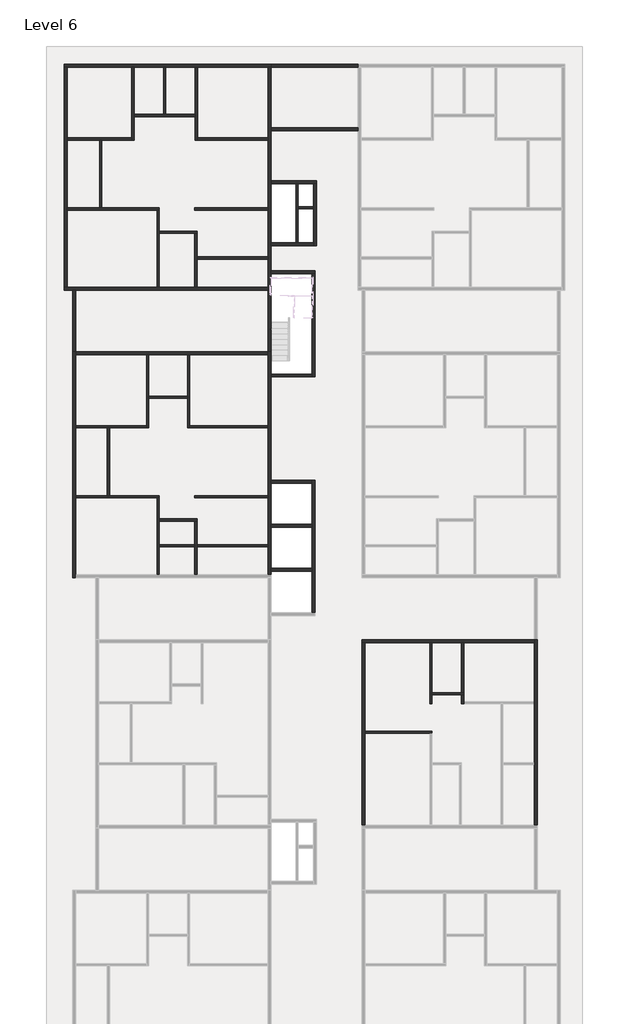
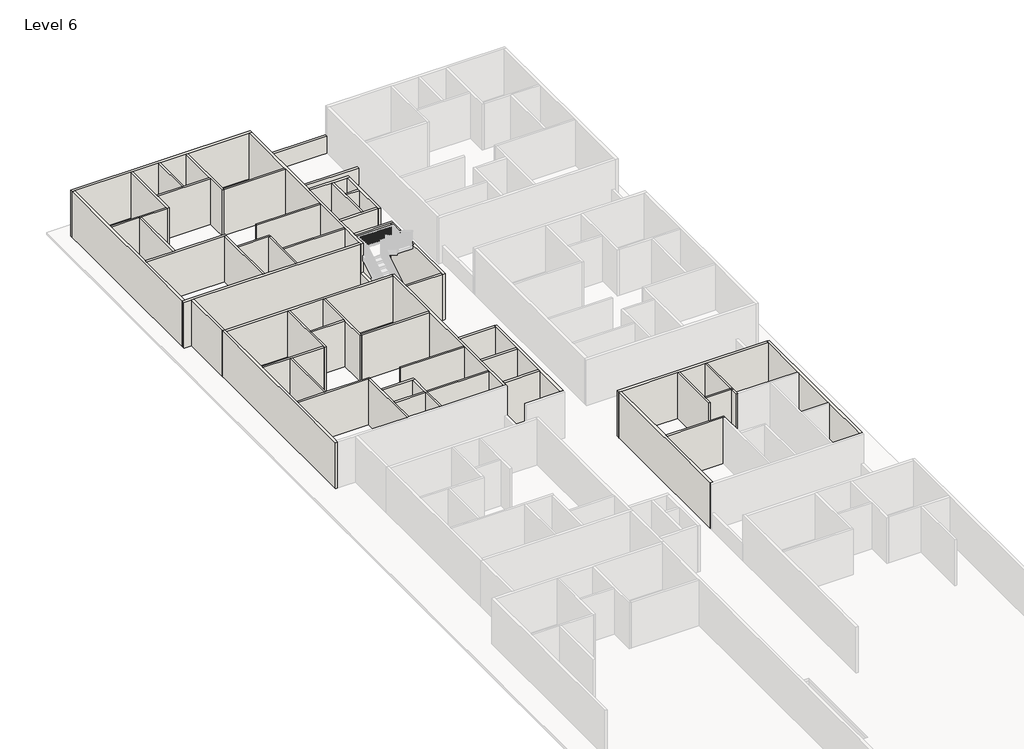
# One storey, part 3 of 8: 57 walls.
"""IFC4 building model written with IfcOpenShell, lengths in millimetres."""

from ifc_helpers import new_model, si_unit, frame, origin, place, context, project, spatial, polyline, outline, extrude, faceted_brep, element, save

model = new_model("IFC4")

# Units and contexts
model_context = context("Model", 3, world=origin())
ifc_project = project(units=[si_unit("LENGTHUNIT", "METRE", prefix="MILLI")], contexts=[model_context])

# Site, building, storey
site = spatial("IfcSite", under=ifc_project)
building = spatial("IfcBuilding", under=site)
storey = spatial("IfcBuildingStorey", under=building, Name="Level 6", Elevation=40474.6172466)

# Walls
placement = place(None, origin())
element("IfcWall", 1, ObjectType="4.5\"", at=placement, inside=storey, context=model_context, shape_type="Brep", body=[
    faceted_brep([(-10818.3415084, 35031.1216096, 40474.6172466), (-10818.3415084, 31373.5216096, 40474.6172466), (-10818.3415084, 31259.2216096, 40474.6172466), (-10818.3415084, 31259.2216096, 43522.6172466), (-10818.3415084, 31373.5216096, 43522.6172466), (-10818.3415084, 35031.1216096, 43522.6172466), (-10704.0415084, 35031.1216096, 40474.6172466), (-10704.0415084, 35031.1216096, 43522.6172466), (-10704.0415084, 32592.7216096, 43522.6172466), (-10704.0415084, 32478.4216096, 43522.6172466), (-10704.0415084, 31259.2216096, 43522.6172466), (-10704.0415084, 31259.2216096, 40474.6172466), (-10704.0415084, 32478.4216096, 40474.6172466), (-10704.0415084, 32592.7216096, 40474.6172466)], [[[0, 1, 2, 3, 4, 5]], [[6, 7, 8, 9, 10, 11, 12, 13]], [[2, 1, 0, 6, 13, 12, 11]], [[0, 5, 7, 6]], [[3, 2, 11, 10]], [[5, 4, 3, 10, 9, 8, 7]]]),
])
element("IfcWall", 2, ObjectType="4.5\"", at=placement, inside=storey, context=model_context, shape_type="Brep", body=[
    faceted_brep([(-10818.3415084, 31373.5216096, 40474.6172466), (-14171.1415084, 31373.5216096, 40474.6172466), (-14171.1415084, 31373.5216096, 43522.6172466), (-10818.3415084, 31373.5216096, 43522.6172466), (-10818.3415084, 31259.2216096, 40474.6172466), (-10818.3415084, 31259.2216096, 43522.6172466), (-12380.4415084, 31259.2216096, 43522.6172466), (-12494.7415084, 31259.2216096, 43522.6172466), (-14171.1415084, 31259.2216096, 43522.6172466), (-14171.1415084, 31259.2216096, 40474.6172466), (-12494.7415084, 31259.2216096, 40474.6172466), (-12380.4415084, 31259.2216096, 40474.6172466)], [[[0, 1, 2, 3]], [[4, 5, 6, 7, 8, 9, 10, 11]], [[1, 0, 4, 11, 10, 9]], [[0, 3, 5, 4]], [[2, 1, 9, 8]], [[3, 2, 8, 7, 6, 5]]]),
])
element("IfcWall", 3, ObjectType="4.5\"", at=placement, inside=storey, context=model_context, shape_type="SweptSolid", body=[
    extrude(outline(polyline([(-12494.7415084, 27754.0216096), (-12494.7415084, 31259.2216096), (-12380.4415084, 31259.2216096), (-12380.4415084, 27754.0216096), (-12494.7415084, 27754.0216096)])), frame((0.0, 0.0, 40474.6172466), z_axis=(0.0, 0.0, 1.0), x_axis=(1.0, 0.0, 0.0)), (0.0, 0.0, 1.0), 3048.0),
])
element("IfcWall", 4, ObjectType="4.5\"", at=placement, inside=storey, context=model_context, shape_type="Brep", body=[
    faceted_brep([(-14171.1415084, 27639.7216096, 40474.6172466), (-9510.2415084, 27639.7216096, 40474.6172466), (-9395.9415084, 27639.7216096, 40474.6172466), (-9395.9415084, 27639.7216096, 43522.6172466), (-9510.2415084, 27639.7216096, 43522.6172466), (-14171.1415084, 27639.7216096, 43522.6172466), (-14171.1415084, 27754.0216096, 40474.6172466), (-14171.1415084, 27754.0216096, 43522.6172466), (-12494.7415084, 27754.0216096, 43522.6172466), (-12380.4415084, 27754.0216096, 43522.6172466), (-9395.9415084, 27754.0216096, 43522.6172466), (-9395.9415084, 27754.0216096, 40474.6172466), (-12380.4415084, 27754.0216096, 40474.6172466), (-12494.7415084, 27754.0216096, 40474.6172466)], [[[0, 1, 2, 3, 4, 5]], [[6, 7, 8, 9, 10, 11, 12, 13]], [[2, 1, 0, 6, 13, 12, 11]], [[0, 5, 7, 6]], [[3, 2, 11, 10]], [[5, 4, 3, 10, 9, 8, 7]]]),
])
element("IfcWall", 5, ObjectType="4.5\"", at=placement, inside=storey, context=model_context, shape_type="Brep", body=[
    faceted_brep([(-9510.2415084, 27639.7216096, 40474.6172466), (-9510.2415084, 23651.9216096, 40474.6172466), (-9510.2415084, 23651.9216096, 43522.6172466), (-9510.2415084, 27639.7216096, 43522.6172466), (-9395.9415084, 27639.7216096, 40474.6172466), (-9395.9415084, 27639.7216096, 43522.6172466), (-9395.9415084, 26547.5216096, 43522.6172466), (-9395.9415084, 26433.2216096, 43522.6172466), (-9395.9415084, 23651.9216096, 43522.6172466), (-9395.9415084, 23651.9216096, 40474.6172466), (-9395.9415084, 26433.2216096, 40474.6172466), (-9395.9415084, 26547.5216096, 40474.6172466)], [[[0, 1, 2, 3]], [[4, 5, 6, 7, 8, 9, 10, 11]], [[1, 0, 4, 11, 10, 9]], [[0, 3, 5, 4]], [[2, 1, 9, 8]], [[3, 2, 8, 7, 6, 5]]]),
])
element("IfcWall", 6, ObjectType="4.5\"", at=placement, inside=storey, context=model_context, shape_type="Brep", body=[
    faceted_brep([(-9395.9415084, 26433.2216096, 40474.6172466), (-7567.1415084, 26433.2216096, 40474.6172466), (-7452.8415084, 26433.2216096, 40474.6172466), (-7452.8415084, 26433.2216096, 43522.6172466), (-7567.1415084, 26433.2216096, 43522.6172466), (-9395.9415084, 26433.2216096, 43522.6172466), (-9395.9415084, 26547.5216096, 40474.6172466), (-9395.9415084, 26547.5216096, 43522.6172466), (-7452.8415084, 26547.5216096, 43522.6172466), (-7452.8415084, 26547.5216096, 40474.6172466)], [[[0, 1, 2, 3, 4, 5]], [[6, 7, 8, 9]], [[2, 1, 0, 6, 9]], [[0, 5, 7, 6]], [[3, 2, 9, 8]], [[5, 4, 3, 8, 7]]]),
])
element("IfcWall", 7, ObjectType="4.5\"", at=placement, inside=storey, context=model_context, shape_type="Brep", body=[
    faceted_brep([(-7567.1415084, 26433.2216096, 40474.6172466), (-7567.1415084, 23651.9216096, 40474.6172466), (-7567.1415084, 23651.9216096, 43522.6172466), (-7567.1415084, 26433.2216096, 43522.6172466), (-7452.8415084, 26433.2216096, 40474.6172466), (-7452.8415084, 26433.2216096, 43522.6172466), (-7452.8415084, 25214.0216096, 43522.6172466), (-7452.8415084, 25099.7216096, 43522.6172466), (-7452.8415084, 23651.9216096, 43522.6172466), (-7452.8415084, 23651.9216096, 40474.6172466), (-7452.8415084, 25099.7216096, 40474.6172466), (-7452.8415084, 25214.0216096, 40474.6172466)], [[[0, 1, 2, 3]], [[4, 5, 6, 7, 8, 9, 10, 11]], [[1, 0, 4, 11, 10, 9]], [[0, 3, 5, 4]], [[2, 1, 9, 8]], [[3, 2, 8, 7, 6, 5]]]),
])
element("IfcWall", 8, ObjectType="4.5\"", at=placement, inside=storey, context=model_context, shape_type="SweptSolid", body=[
    extrude(outline(polyline([(-7452.8415084, 25214.0216096), (-3769.8415084, 25214.0216096), (-3769.8415084, 25099.7216096), (-7452.8415084, 25099.7216096), (-7452.8415084, 25214.0216096)])), frame((0.0, 0.0, 40474.6172466), z_axis=(0.0, 0.0, 1.0), x_axis=(1.0, 0.0, 0.0)), (0.0, 0.0, 1.0), 3048.0),
])
element("IfcWall", 9, ObjectType="4.5\"", at=placement, inside=storey, context=model_context, shape_type="SweptSolid", body=[
    extrude(outline(polyline([(-3769.8415084, 27639.7216096), (-7567.1415084, 27639.7216096), (-7567.1415084, 27754.0216096), (-3769.8415084, 27754.0216096), (-3769.8415084, 27639.7216096)])), frame((0.0, 0.0, 40474.6172466), z_axis=(0.0, 0.0, 1.0), x_axis=(1.0, 0.0, 0.0)), (0.0, 0.0, 1.0), 3048.0),
])
element("IfcWall", 10, ObjectType="4.5\"", at=placement, inside=storey, context=model_context, shape_type="Brep", body=[
    faceted_brep([(-10704.0415084, 32478.4216096, 40474.6172466), (-7541.7415084, 32478.4216096, 40474.6172466), (-7541.7415084, 32478.4216096, 43522.6172466), (-10704.0415084, 32478.4216096, 43522.6172466), (-10704.0415084, 32592.7216096, 40474.6172466), (-10704.0415084, 32592.7216096, 43522.6172466), (-9180.0415084, 32592.7216096, 43522.6172466), (-9065.7415084, 32592.7216096, 43522.6172466), (-7541.7415084, 32592.7216096, 43522.6172466), (-7541.7415084, 32592.7216096, 40474.6172466), (-9065.7415084, 32592.7216096, 40474.6172466), (-9180.0415084, 32592.7216096, 40474.6172466)], [[[0, 1, 2, 3]], [[4, 5, 6, 7, 8, 9, 10, 11]], [[1, 0, 4, 11, 10, 9]], [[0, 3, 5, 4]], [[2, 1, 9, 8]], [[3, 2, 8, 7, 6, 5]]]),
])
element("IfcWall", 11, ObjectType="4.5\"", at=placement, inside=storey, context=model_context, shape_type="SweptSolid", body=[
    extrude(outline(polyline([(-9180.0415084, 32592.7216096), (-9180.0415084, 35031.1216096), (-9065.7415084, 35031.1216096), (-9065.7415084, 32592.7216096), (-9180.0415084, 32592.7216096)])), frame((0.0, 0.0, 40474.6172466), z_axis=(0.0, 0.0, 1.0), x_axis=(1.0, 0.0, 0.0)), (0.0, 0.0, 1.0), 3048.0),
])
element("IfcWall", 12, ObjectType="4.5\"", at=placement, inside=storey, context=model_context, shape_type="Brep", body=[
    faceted_brep([(-7541.7415084, 35031.1216096, 40474.6172466), (-7541.7415084, 32592.7216096, 40474.6172466), (-7541.7415084, 32478.4216096, 40474.6172466), (-7541.7415084, 31259.2216096, 40474.6172466), (-7541.7415084, 31259.2216096, 43522.6172466), (-7541.7415084, 32478.4216096, 43522.6172466), (-7541.7415084, 32592.7216096, 43522.6172466), (-7541.7415084, 35031.1216096, 43522.6172466), (-7427.4415084, 35031.1216096, 40474.6172466), (-7427.4415084, 35031.1216096, 43522.6172466), (-7427.4415084, 31373.5216096, 43522.6172466), (-7427.4415084, 31259.2216096, 43522.6172466), (-7427.4415084, 31259.2216096, 40474.6172466), (-7427.4415084, 31373.5216096, 40474.6172466)], [[[0, 1, 2, 3, 4, 5, 6, 7]], [[8, 9, 10, 11, 12, 13]], [[3, 2, 1, 0, 8, 13, 12]], [[0, 7, 9, 8]], [[4, 3, 12, 11]], [[7, 6, 5, 4, 11, 10, 9]]]),
])
element("IfcWall", 13, ObjectType="4.5\"", at=placement, inside=storey, context=model_context, shape_type="SweptSolid", body=[
    extrude(outline(polyline([(-3769.8415084, 31259.2216096), (-7427.4415084, 31259.2216096), (-7427.4415084, 31373.5216096), (-3769.8415084, 31373.5216096), (-3769.8415084, 31259.2216096)])), frame((0.0, 0.0, 40474.6172466), z_axis=(0.0, 0.0, 1.0), x_axis=(1.0, 0.0, 0.0)), (0.0, 0.0, 1.0), 3048.0),
])
element("IfcWall", 14, ObjectType="4.5\"", at=placement, inside=storey, context=model_context, shape_type="Brep", body=[
    faceted_brep([(-10061.4044854, 20146.7216096, 40474.6172466), (-10061.4044854, 16489.1216096, 40474.6172466), (-10061.4044854, 16374.8216096, 40474.6172466), (-10061.4044854, 16374.8216096, 43522.6172466), (-10061.4044854, 16489.1216096, 43522.6172466), (-10061.4044854, 20146.7216096, 43522.6172466), (-9947.1044854, 20146.7216096, 40474.6172466), (-9947.1044854, 20146.7216096, 43522.6172466), (-9947.1044854, 18013.1216096, 43522.6172466), (-9947.1044854, 17898.8216096, 43522.6172466), (-9947.1044854, 16374.8216096, 43522.6172466), (-9947.1044854, 16374.8216096, 40474.6172466), (-9947.1044854, 17898.8216096, 40474.6172466), (-9947.1044854, 18013.1216096, 40474.6172466)], [[[0, 1, 2, 3, 4, 5]], [[6, 7, 8, 9, 10, 11, 12, 13]], [[2, 1, 0, 6, 13, 12, 11]], [[0, 5, 7, 6]], [[3, 2, 11, 10]], [[5, 4, 3, 10, 9, 8, 7]]]),
])
element("IfcWall", 15, ObjectType="4.5\"", at=placement, inside=storey, context=model_context, shape_type="Brep", body=[
    faceted_brep([(-10061.4044854, 16489.1216096, 40474.6172466), (-13719.0044854, 16489.1216096, 40474.6172466), (-13719.0044854, 16489.1216096, 43522.6172466), (-10061.4044854, 16489.1216096, 43522.6172466), (-10061.4044854, 16374.8216096, 40474.6172466), (-10061.4044854, 16374.8216096, 43522.6172466), (-11980.3915084, 16374.8216096, 43522.6172466), (-12094.6915084, 16374.8216096, 43522.6172466), (-13719.0044854, 16374.8216096, 43522.6172466), (-13719.0044854, 16374.8216096, 40474.6172466), (-12094.6915084, 16374.8216096, 40474.6172466), (-11980.3915084, 16374.8216096, 40474.6172466)], [[[0, 1, 2, 3]], [[4, 5, 6, 7, 8, 9, 10, 11]], [[1, 0, 4, 11, 10, 9]], [[0, 3, 5, 4]], [[2, 1, 9, 8]], [[3, 2, 8, 7, 6, 5]]]),
])
element("IfcWall", 16, ObjectType="4.5\"", at=placement, inside=storey, context=model_context, shape_type="SweptSolid", body=[
    extrude(outline(polyline([(-7940.5044854, 17898.8216096), (-9947.1044854, 17898.8216096), (-9947.1044854, 18013.1216096), (-7940.5044854, 18013.1216096), (-7940.5044854, 17898.8216096)])), frame((0.0, 0.0, 40474.6172466), z_axis=(0.0, 0.0, 1.0), x_axis=(1.0, 0.0, 0.0)), (0.0, 0.0, 1.0), 3048.0),
])
element("IfcWall", 17, ObjectType="4.5\"", at=placement, inside=storey, context=model_context, shape_type="Brep", body=[
    faceted_brep([(-7940.5044854, 20146.7216096, 40474.6172466), (-7940.5044854, 18013.1216096, 40474.6172466), (-7940.5044854, 17898.8216096, 40474.6172466), (-7940.5044854, 16374.8216096, 40474.6172466), (-7940.5044854, 16374.8216096, 43522.6172466), (-7940.5044854, 17898.8216096, 43522.6172466), (-7940.5044854, 18013.1216096, 43522.6172466), (-7940.5044854, 20146.7216096, 43522.6172466), (-7826.2044854, 20146.7216096, 40474.6172466), (-7826.2044854, 20146.7216096, 43522.6172466), (-7826.2044854, 16489.1216096, 43522.6172466), (-7826.2044854, 16374.8216096, 43522.6172466), (-7826.2044854, 16374.8216096, 40474.6172466), (-7826.2044854, 16489.1216096, 40474.6172466)], [[[0, 1, 2, 3, 4, 5, 6, 7]], [[8, 9, 10, 11, 12, 13]], [[3, 2, 1, 0, 8, 13, 12]], [[0, 7, 9, 8]], [[4, 3, 12, 11]], [[7, 6, 5, 4, 11, 10, 9]]]),
])
element("IfcWall", 18, ObjectType="4.5\"", at=placement, inside=storey, context=model_context, shape_type="SweptSolid", body=[
    extrude(outline(polyline([(-3769.8415084, 16374.8216096), (-7826.2044854, 16374.8216096), (-7826.2044854, 16489.1216096), (-3769.8415084, 16489.1216096), (-3769.8415084, 16374.8216096)])), frame((0.0, 0.0, 40474.6172466), z_axis=(0.0, 0.0, 1.0), x_axis=(1.0, 0.0, 0.0)), (0.0, 0.0, 1.0), 3048.0),
])
element("IfcWall", 19, ObjectType="4.5\"", at=placement, inside=storey, context=model_context, shape_type="SweptSolid", body=[
    extrude(outline(polyline([(-12094.6915084, 12869.6216096), (-12094.6915084, 16374.8216096), (-11980.3915084, 16374.8216096), (-11980.3915084, 12869.6216096), (-12094.6915084, 12869.6216096)])), frame((0.0, 0.0, 40474.6172466), z_axis=(0.0, 0.0, 1.0), x_axis=(1.0, 0.0, 0.0)), (0.0, 0.0, 1.0), 3048.0),
])
element("IfcWall", 20, ObjectType="4.5\"", at=placement, inside=storey, context=model_context, shape_type="Brep", body=[
    faceted_brep([(-13719.0044854, 12755.3216096, 40474.6172466), (-9510.2415084, 12755.3216096, 40474.6172466), (-9395.9415084, 12755.3216096, 40474.6172466), (-9395.9415084, 12755.3216096, 43522.6172466), (-9510.2415084, 12755.3216096, 43522.6172466), (-13719.0044854, 12755.3216096, 43522.6172466), (-13719.0044854, 12869.6216096, 40474.6172466), (-13719.0044854, 12869.6216096, 43522.6172466), (-12094.6915084, 12869.6216096, 43522.6172466), (-11980.3915084, 12869.6216096, 43522.6172466), (-9395.9415084, 12869.6216096, 43522.6172466), (-9395.9415084, 12869.6216096, 40474.6172466), (-11980.3915084, 12869.6216096, 40474.6172466), (-12094.6915084, 12869.6216096, 40474.6172466)], [[[0, 1, 2, 3, 4, 5]], [[6, 7, 8, 9, 10, 11, 12, 13]], [[2, 1, 0, 6, 13, 12, 11]], [[0, 5, 7, 6]], [[3, 2, 11, 10]], [[5, 4, 3, 10, 9, 8, 7]]]),
])
element("IfcWall", 21, ObjectType="4.5\"", at=placement, inside=storey, context=model_context, shape_type="Brep", body=[
    faceted_brep([(-9510.2415084, 12755.3216096, 40474.6172466), (-9510.2415084, 8767.5216096, 40474.6172466), (-9510.2415084, 8767.5216096, 43522.6172466), (-9510.2415084, 12755.3216096, 43522.6172466), (-9395.9415084, 12755.3216096, 40474.6172466), (-9395.9415084, 12755.3216096, 43522.6172466), (-9395.9415084, 11663.1216096, 43522.6172466), (-9395.9415084, 11548.8216096, 43522.6172466), (-9395.9415084, 10329.6216096, 43522.6172466), (-9395.9415084, 10215.3216096, 43522.6172466), (-9395.9415084, 8767.5216096, 43522.6172466), (-9395.9415084, 8767.5216096, 40474.6172466), (-9395.9415084, 10215.3216096, 40474.6172466), (-9395.9415084, 10329.6216096, 40474.6172466), (-9395.9415084, 11548.8216096, 40474.6172466), (-9395.9415084, 11663.1216096, 40474.6172466)], [[[0, 1, 2, 3]], [[4, 5, 6, 7, 8, 9, 10, 11, 12, 13, 14, 15]], [[1, 0, 4, 15, 14, 13, 12, 11]], [[0, 3, 5, 4]], [[2, 1, 11, 10]], [[3, 2, 10, 9, 8, 7, 6, 5]]]),
])
element("IfcWall", 22, ObjectType="4.5\"", at=placement, inside=storey, context=model_context, shape_type="SweptSolid", body=[
    extrude(outline(polyline([(-7567.1415084, 10215.3216096), (-9395.9415084, 10215.3216096), (-9395.9415084, 10329.6216096), (-7567.1415084, 10329.6216096), (-7567.1415084, 10215.3216096)])), frame((0.0, 0.0, 40474.6172466), z_axis=(0.0, 0.0, 1.0), x_axis=(1.0, 0.0, 0.0)), (0.0, 0.0, 1.0), 3048.0),
])
element("IfcWall", 23, ObjectType="4.5\"", at=placement, inside=storey, context=model_context, shape_type="Brep", body=[
    faceted_brep([(-9395.9415084, 11548.8216096, 40474.6172466), (-7567.1415084, 11548.8216096, 40474.6172466), (-7452.8415084, 11548.8216096, 40474.6172466), (-7452.8415084, 11548.8216096, 43522.6172466), (-7567.1415084, 11548.8216096, 43522.6172466), (-9395.9415084, 11548.8216096, 43522.6172466), (-9395.9415084, 11663.1216096, 40474.6172466), (-9395.9415084, 11663.1216096, 43522.6172466), (-7452.8415084, 11663.1216096, 43522.6172466), (-7452.8415084, 11663.1216096, 40474.6172466)], [[[0, 1, 2, 3, 4, 5]], [[6, 7, 8, 9]], [[2, 1, 0, 6, 9]], [[0, 5, 7, 6]], [[3, 2, 9, 8]], [[5, 4, 3, 8, 7]]]),
])
element("IfcWall", 24, ObjectType="4.5\"", at=placement, inside=storey, context=model_context, shape_type="Brep", body=[
    faceted_brep([(-7567.1415084, 11548.8216096, 40474.6172466), (-7567.1415084, 10329.6216096, 40474.6172466), (-7567.1415084, 10215.3216096, 40474.6172466), (-7567.1415084, 8767.5216096, 40474.6172466), (-7567.1415084, 8767.5216096, 43522.6172466), (-7567.1415084, 10215.3216096, 43522.6172466), (-7567.1415084, 10329.6216096, 43522.6172466), (-7567.1415084, 11548.8216096, 43522.6172466), (-7452.8415084, 11548.8216096, 40474.6172466), (-7452.8415084, 11548.8216096, 43522.6172466), (-7452.8415084, 10329.6216096, 43522.6172466), (-7452.8415084, 10215.3216096, 43522.6172466), (-7452.8415084, 8767.5216096, 43522.6172466), (-7452.8415084, 8767.5216096, 40474.6172466), (-7452.8415084, 10215.3216096, 40474.6172466), (-7452.8415084, 10329.6216096, 40474.6172466)], [[[0, 1, 2, 3, 4, 5, 6, 7]], [[8, 9, 10, 11, 12, 13, 14, 15]], [[3, 2, 1, 0, 8, 15, 14, 13]], [[0, 7, 9, 8]], [[4, 3, 13, 12]], [[7, 6, 5, 4, 12, 11, 10, 9]]]),
])
element("IfcWall", 25, ObjectType="4.5\"", at=placement, inside=storey, context=model_context, shape_type="SweptSolid", body=[
    extrude(outline(polyline([(-3769.8415084, 10215.3216096), (-7452.8415084, 10215.3216096), (-7452.8415084, 10329.6216096), (-3769.8415084, 10329.6216096), (-3769.8415084, 10215.3216096)])), frame((0.0, 0.0, 40474.6172466), z_axis=(0.0, 0.0, 1.0), x_axis=(1.0, 0.0, 0.0)), (0.0, 0.0, 1.0), 3048.0),
])
element("IfcWall", 26, ObjectType="4.5\"", at=placement, inside=storey, context=model_context, shape_type="SweptSolid", body=[
    extrude(outline(polyline([(-3769.8415084, 12755.3216096), (-7567.1415084, 12755.3216096), (-7567.1415084, 12869.6216096), (-3769.8415084, 12869.6216096), (-3769.8415084, 12755.3216096)])), frame((0.0, 0.0, 40474.6172466), z_axis=(0.0, 0.0, 1.0), x_axis=(1.0, 0.0, 0.0)), (0.0, 0.0, 1.0), 3048.0),
])
element("IfcWall", 27, ObjectType="4.5\"", at=placement, inside=storey, context=model_context, shape_type="Brep", body=[
    faceted_brep([(1259.3584916, 572.7745083, 40474.6172466), (4610.8714687, 572.7745083, 40474.6172466), (4725.1714687, 572.7745083, 40474.6172466), (4725.1714687, 572.7745083, 43522.6172466), (4610.8714687, 572.7745083, 43522.6172466), (1259.3584916, 572.7745083, 43522.6172466), (1259.3584916, 687.0745083, 40474.6172466), (1259.3584916, 687.0745083, 43522.6172466), (4725.1714687, 687.0745083, 43522.6172466), (4725.1714687, 687.0745083, 40474.6172466)], [[[0, 1, 2, 3, 4, 5]], [[6, 7, 8, 9]], [[2, 1, 0, 6, 9]], [[0, 5, 7, 6]], [[3, 2, 9, 8]], [[5, 4, 3, 8, 7]]]),
])
element("IfcWall", 28, ObjectType="4.5\"", at=placement, inside=storey, context=model_context, shape_type="Brep", body=[
    faceted_brep([(4610.8714687, 5262.3216096, 40474.6172466), (4610.8714687, 2100.0216096, 40474.6172466), (4610.8714687, 2100.0216096, 43522.6172466), (4610.8714687, 5262.3216096, 43522.6172466), (4725.1714687, 5262.3216096, 40474.6172466), (4725.1714687, 5262.3216096, 43522.6172466), (4725.1714687, 2671.5216096, 43522.6172466), (4725.1714687, 2557.2216096, 43522.6172466), (4725.1714687, 2100.0216096, 43522.6172466), (4725.1714687, 2100.0216096, 40474.6172466), (4725.1714687, 2557.2216096, 40474.6172466), (4725.1714687, 2671.5216096, 40474.6172466)], [[[0, 1, 2, 3]], [[4, 5, 6, 7, 8, 9, 10, 11]], [[1, 0, 4, 11, 10, 9]], [[2, 1, 9, 8]], [[0, 3, 5, 4]], [[3, 2, 8, 7, 6, 5]]]),
])
element("IfcWall", 29, ObjectType="4.5\"", at=placement, inside=storey, context=model_context, shape_type="Brep", body=[
    faceted_brep([(4725.1714687, 2557.2216096, 40474.6172466), (6249.1714687, 2557.2216096, 40474.6172466), (6363.4714687, 2557.2216096, 40474.6172466), (6363.4714687, 2557.2216096, 43522.6172466), (6249.1714687, 2557.2216096, 43522.6172466), (4725.1714687, 2557.2216096, 43522.6172466), (4725.1714687, 2671.5216096, 40474.6172466), (4725.1714687, 2671.5216096, 43522.6172466), (6249.1714687, 2671.5216096, 43522.6172466), (6363.4714687, 2671.5216096, 43522.6172466), (6363.4714687, 2671.5216096, 40474.6172466), (6249.1714687, 2671.5216096, 40474.6172466)], [[[0, 1, 2, 3, 4, 5]], [[6, 7, 8, 9, 10, 11]], [[2, 1, 0, 6, 11, 10]], [[0, 5, 7, 6]], [[3, 2, 10, 9]], [[5, 4, 3, 9, 8, 7]]]),
])
element("IfcWall", 30, ObjectType="4.5\"", at=placement, inside=storey, context=model_context, shape_type="SweptSolid", body=[
    extrude(outline(polyline([(6363.4714687, 5262.3216096), (6363.4714687, 2671.5216096), (6249.1714687, 2671.5216096), (6249.1714687, 5262.3216096), (6363.4714687, 5262.3216096)])), frame((0.0, 0.0, 40474.6172466), z_axis=(0.0, 0.0, 1.0), x_axis=(1.0, 0.0, 0.0)), (0.0, 0.0, 1.0), 3048.0),
])
element("IfcWall", 31, ObjectType="4.5\"", at=placement, inside=storey, context=model_context, shape_type="Brep", body=[
    faceted_brep([(6249.1714687, 2557.2216096, 40474.6172466), (6249.1714687, 2100.0216096, 40474.6172466), (6249.1714687, 2100.0216096, 43522.6172466), (6249.1714687, 2557.2216096, 43522.6172466), (6363.4714687, 2557.2216096, 40474.6172466), (6363.4714687, 2557.2216096, 43522.6172466), (6363.4714687, 2214.3216096, 43522.6172466), (6363.4714687, 2100.0216096, 43522.6172466), (6363.4714687, 2100.0216096, 40474.6172466), (6363.4714687, 2214.3216096, 40474.6172466)], [[[0, 1, 2, 3]], [[4, 5, 6, 7, 8, 9]], [[1, 0, 4, 9, 8]], [[0, 3, 5, 4]], [[2, 1, 8, 7]], [[3, 2, 7, 6, 5]]]),
])
element("IfcWall", 32, ObjectType="4.5\"", at=placement, inside=storey, context=model_context, shape_type="Brep", body=[
    faceted_brep([(-2321.9738684, 29000.0900967, 40474.6172466), (-2321.9738684, 25952.0900967, 40474.6172466), (-2321.9738684, 25952.0900967, 43522.6172466), (-2321.9738684, 29000.0900967, 43522.6172466), (-2207.6738684, 29000.0900967, 40474.6172466), (-2207.6738684, 29000.0900967, 43522.6172466), (-2207.6738684, 27820.8172885, 43522.6172466), (-2207.6738684, 27706.5172885, 43522.6172466), (-2207.6738684, 25952.0900967, 43522.6172466), (-2207.6738684, 25952.0900967, 40474.6172466), (-2207.6738684, 27706.5172885, 40474.6172466), (-2207.6738684, 27820.8172885, 40474.6172466)], [[[0, 1, 2, 3]], [[4, 5, 6, 7, 8, 9, 10, 11]], [[1, 0, 4, 11, 10, 9]], [[3, 2, 8, 7, 6, 5]], [[0, 3, 5, 4]], [[2, 1, 9, 8]]]),
])
element("IfcWall", 33, ObjectType="4.5\"", at=placement, inside=storey, context=model_context, shape_type="SweptSolid", body=[
    extrude(outline(polyline([(-2207.6738684, 27820.8172885), (-1407.6415084, 27820.8172885), (-1407.6415084, 27706.5172885), (-2207.6738684, 27706.5172885), (-2207.6738684, 27820.8172885)])), frame((0.0, 0.0, 40474.6172466), z_axis=(0.0, 0.0, 1.0), x_axis=(1.0, 0.0, 0.0)), (0.0, 0.0, 1.0), 3048.0),
])
element("IfcWall", 34, ObjectType="6\"", at=placement, inside=storey, context=model_context, shape_type="Brep", body=[
    faceted_brep([(-14323.5415084, 35031.1216096, 40474.6172466), (-14171.1415084, 35031.1216096, 40474.6172466), (-10818.3415084, 35031.1216096, 40474.6172466), (-10704.0415084, 35031.1216096, 40474.6172466), (-9180.0415084, 35031.1216096, 40474.6172466), (-9065.7415084, 35031.1216096, 40474.6172466), (-7541.7415084, 35031.1216096, 40474.6172466), (-7427.4415084, 35031.1216096, 40474.6172466), (-3769.8415084, 35031.1216096, 40474.6172466), (-3617.4415084, 35031.1216096, 40474.6172466), (-3617.4415084, 35031.1216096, 43522.6172466), (-3769.8415084, 35031.1216096, 43522.6172466), (-7427.4415084, 35031.1216096, 43522.6172466), (-7541.7415084, 35031.1216096, 43522.6172466), (-9065.7415084, 35031.1216096, 43522.6172466), (-9180.0415084, 35031.1216096, 43522.6172466), (-10704.0415084, 35031.1216096, 43522.6172466), (-10818.3415084, 35031.1216096, 43522.6172466), (-14171.1415084, 35031.1216096, 43522.6172466), (-14323.5415084, 35031.1216096, 43522.6172466), (-14323.5415084, 35183.5216096, 40474.6172466), (-14323.5415084, 35183.5216096, 43522.6172466), (-3617.4415084, 35183.5216096, 43522.6172466), (-3617.4415084, 35183.5216096, 40474.6172466)], [[[0, 1, 2, 3, 4, 5, 6, 7, 8, 9, 10, 11, 12, 13, 14, 15, 16, 17, 18, 19]], [[20, 21, 22, 23]], [[9, 8, 7, 6, 5, 4, 3, 2, 1, 0, 20, 23]], [[0, 19, 21, 20]], [[9, 23, 22, 10]], [[19, 18, 17, 16, 15, 14, 13, 12, 11, 10, 22, 21]]]),
])
element("IfcWall", 35, ObjectType="6\"", at=placement, inside=storey, context=model_context, shape_type="Brep", body=[
    faceted_brep([(-3769.8415084, 35031.1216096, 43522.6172466), (-3769.8415084, 35031.1216096, 40474.6172466), (-3769.8415084, 31373.5216096, 40474.6172466), (-3769.8415084, 31259.2216096, 40474.6172466), (-3769.8415084, 27754.0216096, 40474.6172466), (-3769.8415084, 27639.7216096, 40474.6172466), (-3769.8415084, 25214.0216096, 40474.6172466), (-3769.8415084, 25099.7216096, 40474.6172466), (-3769.8415084, 23651.9216096, 40474.6172466), (-3769.8415084, 23499.5216096, 40474.6172466), (-3769.8415084, 23499.5216096, 43522.6172466), (-3769.8415084, 23651.9216096, 43522.6172466), (-3769.8415084, 25099.7216096, 43522.6172466), (-3769.8415084, 25214.0216096, 43522.6172466), (-3769.8415084, 27639.7216096, 43522.6172466), (-3769.8415084, 27754.0216096, 43522.6172466), (-3769.8415084, 31259.2216096, 43522.6172466), (-3769.8415084, 31373.5216096, 43522.6172466), (-3617.4415084, 35031.1216096, 40474.6172466), (-3617.4415084, 35031.1216096, 43522.6172466), (-3617.4415084, 29152.4900967, 43522.6172466), (-3617.4415084, 29000.0900967, 43522.6172466), (-3617.4415084, 25952.0900967, 43522.6172466), (-3617.4415084, 25799.6900967, 43522.6172466), (-3617.4415084, 24490.1216096, 43522.6172466), (-3617.4415084, 24337.7216096, 43522.6172466), (-3617.4415084, 23499.5216096, 43522.6172466), (-3617.4415084, 23499.5216096, 40474.6172466), (-3617.4415084, 24337.7216096, 40474.6172466), (-3617.4415084, 24490.1216096, 40474.6172466), (-3617.4415084, 25799.6900967, 40474.6172466), (-3617.4415084, 25952.0900967, 40474.6172466), (-3617.4415084, 29000.0900967, 40474.6172466), (-3617.4415084, 29152.4900967, 40474.6172466), (-3617.4415084, 31744.9197155, 40474.6172466), (-3617.4415084, 31897.3197155, 40474.6172466)], [[[0, 1, 2, 3, 4, 5, 6, 7, 8, 9, 10, 11, 12, 13, 14, 15, 16, 17]], [[18, 19, 20, 21, 22, 23, 24, 25, 26, 27, 28, 29, 30, 31, 32, 33, 34, 35]], [[9, 8, 7, 6, 5, 4, 3, 2, 1, 18, 35, 34, 33, 32, 31, 30, 29, 28, 27]], [[0, 19, 18, 1]], [[9, 27, 26, 10]], [[0, 17, 16, 15, 14, 13, 12, 11, 10, 26, 25, 24, 23, 22, 21, 20, 19]]]),
])
element("IfcWall", 36, ObjectType="6\"", at=placement, inside=storey, context=model_context, shape_type="Brep", body=[
    faceted_brep([(-3769.8415084, 23651.9216096, 43522.6172466), (-3769.8415084, 23651.9216096, 40474.6172466), (-7452.8415084, 23651.9216096, 40474.6172466), (-7567.1415084, 23651.9216096, 40474.6172466), (-9395.9415084, 23651.9216096, 40474.6172466), (-9510.2415084, 23651.9216096, 40474.6172466), (-14171.1415084, 23651.9216096, 40474.6172466), (-14323.5415084, 23651.9216096, 40474.6172466), (-14323.5415084, 23651.9216096, 43522.6172466), (-14171.1415084, 23651.9216096, 43522.6172466), (-9510.2415084, 23651.9216096, 43522.6172466), (-9395.9415084, 23651.9216096, 43522.6172466), (-7567.1415084, 23651.9216096, 43522.6172466), (-7452.8415084, 23651.9216096, 43522.6172466), (-3769.8415084, 23499.5216096, 40474.6172466), (-3769.8415084, 23499.5216096, 43522.6172466), (-13719.0044854, 23499.5216096, 43522.6172466), (-13871.4044854, 23499.5216096, 43522.6172466), (-14323.5415084, 23499.5216096, 43522.6172466), (-14323.5415084, 23499.5216096, 40474.6172466), (-13871.4044854, 23499.5216096, 40474.6172466), (-13719.0044854, 23499.5216096, 40474.6172466)], [[[0, 1, 2, 3, 4, 5, 6, 7, 8, 9, 10, 11, 12, 13]], [[14, 15, 16, 17, 18, 19, 20, 21]], [[7, 6, 5, 4, 3, 2, 1, 14, 21, 20, 19]], [[8, 7, 19, 18]], [[0, 15, 14, 1]], [[0, 13, 12, 11, 10, 9, 8, 18, 17, 16, 15]]]),
])
element("IfcWall", 37, ObjectType="6\"", at=placement, inside=storey, context=model_context, shape_type="Brep", body=[
    faceted_brep([(-14171.1415084, 23651.9216096, 40474.6172466), (-14171.1415084, 27639.7216096, 40474.6172466), (-14171.1415084, 27754.0216096, 40474.6172466), (-14171.1415084, 31259.2216096, 40474.6172466), (-14171.1415084, 31373.5216096, 40474.6172466), (-14171.1415084, 35031.1216096, 40474.6172466), (-14171.1415084, 35031.1216096, 43522.6172466), (-14171.1415084, 31373.5216096, 43522.6172466), (-14171.1415084, 31259.2216096, 43522.6172466), (-14171.1415084, 27754.0216096, 43522.6172466), (-14171.1415084, 27639.7216096, 43522.6172466), (-14171.1415084, 23651.9216096, 43522.6172466), (-14323.5415084, 23651.9216096, 40474.6172466), (-14323.5415084, 23651.9216096, 43522.6172466), (-14323.5415084, 35031.1216096, 43522.6172466), (-14323.5415084, 35031.1216096, 40474.6172466)], [[[0, 1, 2, 3, 4, 5, 6, 7, 8, 9, 10, 11]], [[12, 13, 14, 15]], [[5, 4, 3, 2, 1, 0, 12, 15]], [[6, 5, 15, 14]], [[0, 11, 13, 12]], [[11, 10, 9, 8, 7, 6, 14, 13]]]),
])
element("IfcWall", 38, ObjectType="6\"", at=placement, inside=storey, context=model_context, shape_type="Brep", body=[
    faceted_brep([(-13871.4044854, 20299.1216096, 40474.6172466), (-13871.4044854, 8615.1216096, 40474.6172466), (-13871.4044854, 8615.1216096, 43522.6172466), (-13871.4044854, 20299.1216096, 43522.6172466), (-13719.0044854, 20299.1216096, 40474.6172466), (-13719.0044854, 20299.1216096, 43522.6172466), (-13719.0044854, 20146.7216096, 43522.6172466), (-13719.0044854, 16489.1216096, 43522.6172466), (-13719.0044854, 16374.8216096, 43522.6172466), (-13719.0044854, 12869.6216096, 43522.6172466), (-13719.0044854, 12755.3216096, 43522.6172466), (-13719.0044854, 8767.5216096, 43522.6172466), (-13719.0044854, 8615.1216096, 43522.6172466), (-13719.0044854, 8615.1216096, 40474.6172466), (-13719.0044854, 8767.5216096, 40474.6172466), (-13719.0044854, 12755.3216096, 40474.6172466), (-13719.0044854, 12869.6216096, 40474.6172466), (-13719.0044854, 16374.8216096, 40474.6172466), (-13719.0044854, 16489.1216096, 40474.6172466), (-13719.0044854, 20146.7216096, 40474.6172466)], [[[0, 1, 2, 3]], [[4, 5, 6, 7, 8, 9, 10, 11, 12, 13, 14, 15, 16, 17, 18, 19]], [[1, 0, 4, 19, 18, 17, 16, 15, 14, 13]], [[2, 1, 13, 12]], [[0, 3, 5, 4]], [[3, 2, 12, 11, 10, 9, 8, 7, 6, 5]]]),
])
element("IfcWall", 39, ObjectType="6\"", at=placement, inside=storey, context=model_context, shape_type="Brep", body=[
    faceted_brep([(-3617.4415084, 8767.5216096, 43522.6172466), (-3617.4415084, 8767.5216096, 40474.6172466), (-3617.4415084, 8945.2303368, 40474.6172466), (-3617.4415084, 9097.6303368, 40474.6172466), (-3617.4415084, 11231.2303368, 40474.6172466), (-3617.4415084, 11383.6303368, 40474.6172466), (-3617.4415084, 13517.2303368, 40474.6172466), (-3617.4415084, 13669.6303368, 40474.6172466), (-3617.4415084, 19003.7216096, 40474.6172466), (-3617.4415084, 19156.1216096, 40474.6172466), (-3617.4415084, 20299.1216096, 40474.6172466), (-3617.4415084, 20299.1216096, 43522.6172466), (-3617.4415084, 19156.1216096, 43522.6172466), (-3617.4415084, 19003.7216096, 43522.6172466), (-3617.4415084, 13669.6303368, 43522.6172466), (-3617.4415084, 13517.2303368, 43522.6172466), (-3617.4415084, 11383.6303368, 43522.6172466), (-3617.4415084, 11231.2303368, 43522.6172466), (-3617.4415084, 9097.6303368, 43522.6172466), (-3617.4415084, 8945.2303368, 43522.6172466), (-3769.8415084, 8767.5216096, 40474.6172466), (-3769.8415084, 8767.5216096, 43522.6172466), (-3769.8415084, 10215.3216096, 43522.6172466), (-3769.8415084, 10329.6216096, 43522.6172466), (-3769.8415084, 12755.3216096, 43522.6172466), (-3769.8415084, 12869.6216096, 43522.6172466), (-3769.8415084, 16374.8216096, 43522.6172466), (-3769.8415084, 16489.1216096, 43522.6172466), (-3769.8415084, 20146.7216096, 43522.6172466), (-3769.8415084, 20299.1216096, 43522.6172466), (-3769.8415084, 20299.1216096, 40474.6172466), (-3769.8415084, 20146.7216096, 40474.6172466), (-3769.8415084, 16489.1216096, 40474.6172466), (-3769.8415084, 16374.8216096, 40474.6172466), (-3769.8415084, 12869.6216096, 40474.6172466), (-3769.8415084, 12755.3216096, 40474.6172466), (-3769.8415084, 10329.6216096, 40474.6172466), (-3769.8415084, 10215.3216096, 40474.6172466)], [[[0, 1, 2, 3, 4, 5, 6, 7, 8, 9, 10, 11, 12, 13, 14, 15, 16, 17, 18, 19]], [[20, 21, 22, 23, 24, 25, 26, 27, 28, 29, 30, 31, 32, 33, 34, 35, 36, 37]], [[10, 9, 8, 7, 6, 5, 4, 3, 2, 1, 20, 37, 36, 35, 34, 33, 32, 31, 30]], [[10, 30, 29, 11]], [[0, 21, 20, 1]], [[0, 19, 18, 17, 16, 15, 14, 13, 12, 11, 29, 28, 27, 26, 25, 24, 23, 22, 21]]]),
])
element("IfcWall", 40, ObjectType="6\"", at=placement, inside=storey, context=model_context, shape_type="Brep", body=[
    faceted_brep([(-3769.8415084, 20299.1216096, 43522.6172466), (-3769.8415084, 20299.1216096, 40474.6172466), (-13719.0044854, 20299.1216096, 40474.6172466), (-13719.0044854, 20299.1216096, 43522.6172466), (-3769.8415084, 20146.7216096, 40474.6172466), (-3769.8415084, 20146.7216096, 43522.6172466), (-7826.2044854, 20146.7216096, 43522.6172466), (-7940.5044854, 20146.7216096, 43522.6172466), (-9947.1044854, 20146.7216096, 43522.6172466), (-10061.4044854, 20146.7216096, 43522.6172466), (-13719.0044854, 20146.7216096, 43522.6172466), (-13719.0044854, 20146.7216096, 40474.6172466), (-10061.4044854, 20146.7216096, 40474.6172466), (-9947.1044854, 20146.7216096, 40474.6172466), (-7940.5044854, 20146.7216096, 40474.6172466), (-7826.2044854, 20146.7216096, 40474.6172466)], [[[0, 1, 2, 3]], [[4, 5, 6, 7, 8, 9, 10, 11, 12, 13, 14, 15]], [[2, 1, 4, 15, 14, 13, 12, 11]], [[3, 2, 11, 10]], [[0, 5, 4, 1]], [[0, 3, 10, 9, 8, 7, 6, 5]]]),
])
element("IfcWall", 41, ObjectType="6\"", at=placement, inside=storey, context=model_context, shape_type="Brep", body=[
    faceted_brep([(10173.4714687, -4185.9344126, 43522.6172466), (10173.4714687, -4185.9344126, 40474.6172466), (10173.4714687, 5414.7216096, 40474.6172466), (10173.4714687, 5414.7216096, 43522.6172466), (10021.0714687, -4185.9344126, 40474.6172466), (10021.0714687, -4185.9344126, 43522.6172466), (10021.0714687, -1061.7344126, 43522.6172466), (10021.0714687, -947.4344126, 43522.6172466), (10021.0714687, 2100.0216096, 43522.6172466), (10021.0714687, 2214.3216096, 43522.6172466), (10021.0714687, 5262.3216096, 43522.6172466), (10021.0714687, 5414.7216096, 43522.6172466), (10021.0714687, 5414.7216096, 40474.6172466), (10021.0714687, 5262.3216096, 40474.6172466), (10021.0714687, 2214.3216096, 40474.6172466), (10021.0714687, 2100.0216096, 40474.6172466), (10021.0714687, -947.4344126, 40474.6172466), (10021.0714687, -1061.7344126, 40474.6172466)], [[[0, 1, 2, 3]], [[4, 5, 6, 7, 8, 9, 10, 11, 12, 13, 14, 15, 16, 17]], [[2, 1, 4, 17, 16, 15, 14, 13, 12]], [[2, 12, 11, 3]], [[0, 5, 4, 1]], [[0, 3, 11, 10, 9, 8, 7, 6, 5]]]),
])
element("IfcWall", 42, ObjectType="6\"", at=placement, inside=storey, context=model_context, shape_type="Brep", body=[
    faceted_brep([(10021.0714687, 5414.7216096, 43522.6172466), (10021.0714687, 5414.7216096, 40474.6172466), (1106.9584916, 5414.7216096, 40474.6172466), (1106.9584916, 5414.7216096, 43522.6172466), (10021.0714687, 5262.3216096, 40474.6172466), (10021.0714687, 5262.3216096, 43522.6172466), (6363.4714687, 5262.3216096, 43522.6172466), (6249.1714687, 5262.3216096, 43522.6172466), (4725.1714687, 5262.3216096, 43522.6172466), (4610.8714687, 5262.3216096, 43522.6172466), (1259.3584916, 5262.3216096, 43522.6172466), (1106.9584916, 5262.3216096, 43522.6172466), (1106.9584916, 5262.3216096, 40474.6172466), (1259.3584916, 5262.3216096, 40474.6172466), (4610.8714687, 5262.3216096, 40474.6172466), (4725.1714687, 5262.3216096, 40474.6172466), (6249.1714687, 5262.3216096, 40474.6172466), (6363.4714687, 5262.3216096, 40474.6172466)], [[[0, 1, 2, 3]], [[4, 5, 6, 7, 8, 9, 10, 11, 12, 13, 14, 15, 16, 17]], [[2, 1, 4, 17, 16, 15, 14, 13, 12]], [[3, 2, 12, 11]], [[0, 5, 4, 1]], [[0, 3, 11, 10, 9, 8, 7, 6, 5]]]),
])
element("IfcWall", 43, ObjectType="6\"", at=placement, inside=storey, context=model_context, shape_type="Brep", body=[
    faceted_brep([(1106.9584916, 5262.3216096, 40474.6172466), (1106.9584916, -4185.9344126, 40474.6172466), (1106.9584916, -4185.9344126, 43522.6172466), (1106.9584916, 5262.3216096, 43522.6172466), (1259.3584916, 5262.3216096, 40474.6172466), (1259.3584916, 5262.3216096, 43522.6172466), (1259.3584916, 687.0745083, 43522.6172466), (1259.3584916, 572.7745083, 43522.6172466), (1259.3584916, -4185.9344126, 43522.6172466), (1259.3584916, -4185.9344126, 40474.6172466), (1259.3584916, 572.7745083, 40474.6172466), (1259.3584916, 687.0745083, 40474.6172466)], [[[0, 1, 2, 3]], [[4, 5, 6, 7, 8, 9, 10, 11]], [[1, 0, 4, 11, 10, 9]], [[0, 3, 5, 4]], [[1, 9, 8, 2]], [[3, 2, 8, 7, 6, 5]]]),
])
element("IfcWall", 44, ObjectType="6\"", at=placement, inside=storey, context=model_context, shape_type="Brep", body=[
    faceted_brep([(-1331.4415084, 6811.6303368, 40474.6172466), (-1331.4415084, 13669.6303368, 40474.6172466), (-1331.4415084, 13669.6303368, 43522.6172466), (-1331.4415084, 6811.6303368, 43522.6172466), (-1483.8415084, 6811.6303368, 40474.6172466), (-1483.8415084, 6811.6303368, 43522.6172466), (-1483.8415084, 8945.2303368, 43522.6172466), (-1483.8415084, 9097.6303368, 43522.6172466), (-1483.8415084, 11231.2303368, 43522.6172466), (-1483.8415084, 11383.6303368, 43522.6172466), (-1483.8415084, 13517.2303368, 43522.6172466), (-1483.8415084, 13669.6303368, 43522.6172466), (-1483.8415084, 13669.6303368, 40474.6172466), (-1483.8415084, 13517.2303368, 40474.6172466), (-1483.8415084, 11383.6303368, 40474.6172466), (-1483.8415084, 11231.2303368, 40474.6172466), (-1483.8415084, 9097.6303368, 40474.6172466), (-1483.8415084, 8945.2303368, 40474.6172466)], [[[0, 1, 2, 3]], [[4, 5, 6, 7, 8, 9, 10, 11, 12, 13, 14, 15, 16, 17]], [[1, 0, 4, 17, 16, 15, 14, 13, 12]], [[3, 2, 11, 10, 9, 8, 7, 6, 5]], [[0, 3, 5, 4]], [[2, 1, 12, 11]]]),
])
element("IfcWall", 45, ObjectType="6\"", at=placement, inside=storey, context=model_context, shape_type="SweptSolid", body=[
    extrude(outline(polyline([(-3617.4415084, 13669.6303368), (-1483.8415084, 13669.6303368), (-1483.8415084, 13517.2303368), (-3617.4415084, 13517.2303368), (-3617.4415084, 13669.6303368)])), frame((0.0, 0.0, 40474.6172466), z_axis=(0.0, 0.0, 1.0), x_axis=(1.0, 0.0, 0.0)), (0.0, 0.0, 1.0), 3048.0),
])
element("IfcWall", 46, ObjectType="6\"", at=placement, inside=storey, context=model_context, shape_type="SweptSolid", body=[
    extrude(outline(polyline([(-1483.8415084, 8945.2303368), (-3617.4415084, 8945.2303368), (-3617.4415084, 9097.6303368), (-1483.8415084, 9097.6303368), (-1483.8415084, 8945.2303368)])), frame((0.0, 0.0, 40474.6172466), z_axis=(0.0, 0.0, 1.0), x_axis=(1.0, 0.0, 0.0)), (0.0, 0.0, 1.0), 3048.0),
])
element("IfcWall", 47, ObjectType="6\"", at=placement, inside=storey, context=model_context, shape_type="SweptSolid", body=[
    extrude(outline(polyline([(-3617.4415084, 11383.6303368), (-1483.8415084, 11383.6303368), (-1483.8415084, 11231.2303368), (-3617.4415084, 11231.2303368), (-3617.4415084, 11383.6303368)])), frame((0.0, 0.0, 40474.6172466), z_axis=(0.0, 0.0, 1.0), x_axis=(1.0, 0.0, 0.0)), (0.0, 0.0, 1.0), 3048.0),
])
element("IfcWall", 48, ObjectType="6\"", at=placement, inside=storey, context=model_context, shape_type="Brep", body=[
    faceted_brep([(-3617.4415084, 29000.0900967, 40474.6172466), (-2321.9738684, 29000.0900967, 40474.6172466), (-2207.6738684, 29000.0900967, 40474.6172466), (-1407.6415084, 29000.0900967, 40474.6172466), (-1255.2415084, 29000.0900967, 40474.6172466), (-1255.2415084, 29000.0900967, 43522.6172466), (-1407.6415084, 29000.0900967, 43522.6172466), (-2207.6738684, 29000.0900967, 43522.6172466), (-2321.9738684, 29000.0900967, 43522.6172466), (-3617.4415084, 29000.0900967, 43522.6172466), (-3617.4415084, 29152.4900967, 40474.6172466), (-3617.4415084, 29152.4900967, 43522.6172466), (-1255.2415084, 29152.4900967, 43522.6172466), (-1255.2415084, 29152.4900967, 40474.6172466)], [[[0, 1, 2, 3, 4, 5, 6, 7, 8, 9]], [[10, 11, 12, 13]], [[4, 3, 2, 1, 0, 10, 13]], [[9, 8, 7, 6, 5, 12, 11]], [[0, 9, 11, 10]], [[5, 4, 13, 12]]]),
])
element("IfcWall", 49, ObjectType="6\"", at=placement, inside=storey, context=model_context, shape_type="Brep", body=[
    faceted_brep([(-1407.6415084, 29000.0900967, 40474.6172466), (-1407.6415084, 27820.8172885, 40474.6172466), (-1407.6415084, 27706.5172885, 40474.6172466), (-1407.6415084, 25952.0900967, 40474.6172466), (-1407.6415084, 25799.6900967, 40474.6172466), (-1407.6415084, 25799.6900967, 43522.6172466), (-1407.6415084, 25952.0900967, 43522.6172466), (-1407.6415084, 27706.5172885, 43522.6172466), (-1407.6415084, 27820.8172885, 43522.6172466), (-1407.6415084, 29000.0900967, 43522.6172466), (-1255.2415084, 29000.0900967, 40474.6172466), (-1255.2415084, 29000.0900967, 43522.6172466), (-1255.2415084, 25799.6900967, 43522.6172466), (-1255.2415084, 25799.6900967, 40474.6172466)], [[[0, 1, 2, 3, 4, 5, 6, 7, 8, 9]], [[10, 11, 12, 13]], [[4, 3, 2, 1, 0, 10, 13]], [[9, 8, 7, 6, 5, 12, 11]], [[0, 9, 11, 10]], [[5, 4, 13, 12]]]),
])
element("IfcWall", 50, ObjectType="6\"", at=placement, inside=storey, context=model_context, shape_type="Brep", body=[
    faceted_brep([(-1407.6415084, 25952.0900967, 40474.6172466), (-2207.6738684, 25952.0900967, 40474.6172466), (-2321.9738684, 25952.0900967, 40474.6172466), (-3617.4415084, 25952.0900967, 40474.6172466), (-3617.4415084, 25952.0900967, 43522.6172466), (-2321.9738684, 25952.0900967, 43522.6172466), (-2207.6738684, 25952.0900967, 43522.6172466), (-1407.6415084, 25952.0900967, 43522.6172466), (-1407.6415084, 25799.6900967, 40474.6172466), (-1407.6415084, 25799.6900967, 43522.6172466), (-3617.4415084, 25799.6900967, 43522.6172466), (-3617.4415084, 25799.6900967, 40474.6172466)], [[[0, 1, 2, 3, 4, 5, 6, 7]], [[8, 9, 10, 11]], [[3, 2, 1, 0, 8, 11]], [[7, 6, 5, 4, 10, 9]], [[0, 7, 9, 8]], [[4, 3, 11, 10]]]),
])
element("IfcWall", 51, ObjectType="6\"", at=placement, inside=storey, context=model_context, shape_type="Brep", body=[
    faceted_brep([(-3617.4415084, 24337.7216096, 40474.6172466), (-1483.8415084, 24337.7216096, 40474.6172466), (-1331.4415084, 24337.7216096, 40474.6172466), (-1331.4415084, 24337.7216096, 43522.6172466), (-1483.8415084, 24337.7216096, 43522.6172466), (-3617.4415084, 24337.7216096, 43522.6172466), (-3617.4415084, 24490.1216096, 40474.6172466), (-3617.4415084, 24490.1216096, 43522.6172466), (-1331.4415084, 24490.1216096, 43522.6172466), (-1331.4415084, 24490.1216096, 40474.6172466)], [[[0, 1, 2, 3, 4, 5]], [[6, 7, 8, 9]], [[2, 1, 0, 6, 9]], [[5, 4, 3, 8, 7]], [[0, 5, 7, 6]], [[3, 2, 9, 8]]]),
])
element("IfcWall", 52, ObjectType="6\"", at=placement, inside=storey, context=model_context, shape_type="Brep", body=[
    faceted_brep([(-1483.8415084, 24337.7216096, 40474.6172466), (-1483.8415084, 19156.1216096, 40474.6172466), (-1483.8415084, 19003.7216096, 40474.6172466), (-1483.8415084, 19003.7216096, 43522.6172466), (-1483.8415084, 19156.1216096, 43522.6172466), (-1483.8415084, 24337.7216096, 43522.6172466), (-1331.4415084, 24337.7216096, 40474.6172466), (-1331.4415084, 24337.7216096, 43522.6172466), (-1331.4415084, 19003.7216096, 43522.6172466), (-1331.4415084, 19003.7216096, 40474.6172466)], [[[0, 1, 2, 3, 4, 5]], [[6, 7, 8, 9]], [[2, 1, 0, 6, 9]], [[5, 4, 3, 8, 7]], [[0, 5, 7, 6]], [[3, 2, 9, 8]]]),
])
element("IfcWall", 53, ObjectType="6\"", at=placement, inside=storey, context=model_context, shape_type="SweptSolid", body=[
    extrude(outline(polyline([(-3617.4415084, 19156.1216096), (-1483.8415084, 19156.1216096), (-1483.8415084, 19003.7216096), (-3617.4415084, 19003.7216096), (-3617.4415084, 19156.1216096)])), frame((0.0, 0.0, 40474.6172466), z_axis=(0.0, 0.0, 1.0), x_axis=(1.0, 0.0, 0.0)), (0.0, 0.0, 1.0), 3048.0),
])
element("IfcWall", 54, ObjectType="6\" 2", at=placement, inside=storey, context=model_context, shape_type="SweptSolid", body=[
    extrude(outline(polyline([(-13871.4044854, 20299.1216096), (-13871.4044854, 23499.5216096), (-13719.0044854, 23499.5216096), (-13719.0044854, 20299.1216096), (-13871.4044854, 20299.1216096)])), frame((0.0, 0.0, 40474.6172466), z_axis=(0.0, 0.0, 1.0), x_axis=(1.0, 0.0, 0.0)), (0.0, 0.0, 1.0), 3048.0),
])
element("IfcWall", 55, ObjectType="6\" 2", at=placement, inside=storey, context=model_context, shape_type="SweptSolid", body=[
    extrude(outline(polyline([(878.4443719, 35031.1216096), (-3617.4415084, 35031.1216096), (-3617.4415084, 35183.5216096), (878.4443719, 35183.5216096), (878.4443719, 35031.1216096)])), frame((0.0, 0.0, 40474.6172466), z_axis=(0.0, 0.0, 1.0), x_axis=(1.0, 0.0, 0.0)), (0.0, 0.0, 1.0), 1219.2),
])
element("IfcWall", 56, ObjectType="6\" 2", at=placement, inside=storey, context=model_context, shape_type="SweptSolid", body=[
    extrude(outline(polyline([(878.4443719, 31744.9197155), (-3617.4415084, 31744.9197155), (-3617.4415084, 31897.3197155), (878.4443719, 31897.3197155), (878.4443719, 31744.9197155)])), frame((0.0, 0.0, 40474.6172466), z_axis=(0.0, 0.0, 1.0), x_axis=(1.0, 0.0, 0.0)), (0.0, 0.0, 1.0), 1219.2),
])
element("IfcWall", 57, ObjectType="6\" 2", at=placement, inside=storey, context=model_context, shape_type="SweptSolid", body=[
    extrude(outline(polyline([(-3769.8415084, 20299.1216096), (-3769.8415084, 23499.5216096), (-3617.4415084, 23499.5216096), (-3617.4415084, 20299.1216096), (-3769.8415084, 20299.1216096)])), frame((0.0, 0.0, 40474.6172466), z_axis=(0.0, 0.0, 1.0), x_axis=(1.0, 0.0, 0.0)), (0.0, 0.0, 1.0), 1219.2),
])

save(model, "model.ifc")

# Revit data of these elements
# Type "4.5\""
#   Assembly Code = "B2010"
#   Layers, outside or top first: 0' - 4 1/2" "WALLS" (function 1)
# Type "6\""
#   Assembly Code = "B2010"
#   Layers, outside or top first: 0' - 6" "WALLS" (function 1)
# Type "6\" 2"
#   Assembly Code = "B2010"
#   Layers, outside or top first: 0' - 6" "4'" (function 1)
# Elements 1, 2, 3, 4, 5, 6, 7, 8, 9, 10, 11, 12, 13, 14, 15, 16, 17, 18, 19, 20, 21, 22, 23, 24, 25, 26, 27, 28, 29, 30, 31, 32, 33 (IfcWall, "4.5\"")
#   Top Offset = 0' - 0"
#   Base Offset = 0' - 0"
#   Unconnected Height = 10' - 0"
#   wall height = 10' - 0"
#   Phase Created = New Construction
#   Base Constraint = Level 6
#   Materials on its faces: "WALLS"
# Elements 34, 35, 36, 37, 38, 39, 40, 41, 42, 43, 44, 45, 46, 47, 48, 49, 50, 51, 52, 53 (IfcWall, "6\"")
#   Top Offset = 0' - 0"
#   Base Offset = 0' - 0"
#   Unconnected Height = 10' - 0"
#   wall height = 10' - 0"
#   Phase Created = New Construction
#   Base Constraint = Level 6
#   Materials on its faces: "WALLS"
# Element 54 (IfcWall, "6\" 2")
#   Top Offset = 0' - 0"
#   Base Offset = 0' - 0"
#   Unconnected Height = 10' - 0"
#   wall height = 10' - 0"
#   Phase Created = New Construction
#   Base Constraint = Level 6
#   Materials on its faces: "4'"
# Elements 55, 56, 57 (IfcWall, "6\" 2")
#   Top Offset = 0' - 0"
#   Base Offset = 0' - 0"
#   Unconnected Height = 4' - 0"
#   wall height = 4' - 0"
#   Phase Created = New Construction
#   Base Constraint = Level 6
#   Materials on its faces: "4'"
# Materials
#   "WALLS": class "Generic", colour RGB 120 120 120, transparency 0, Cost = 0
#   "4'": class "Generic", colour RGB 120 120 120, transparency 0, Cost = 0
